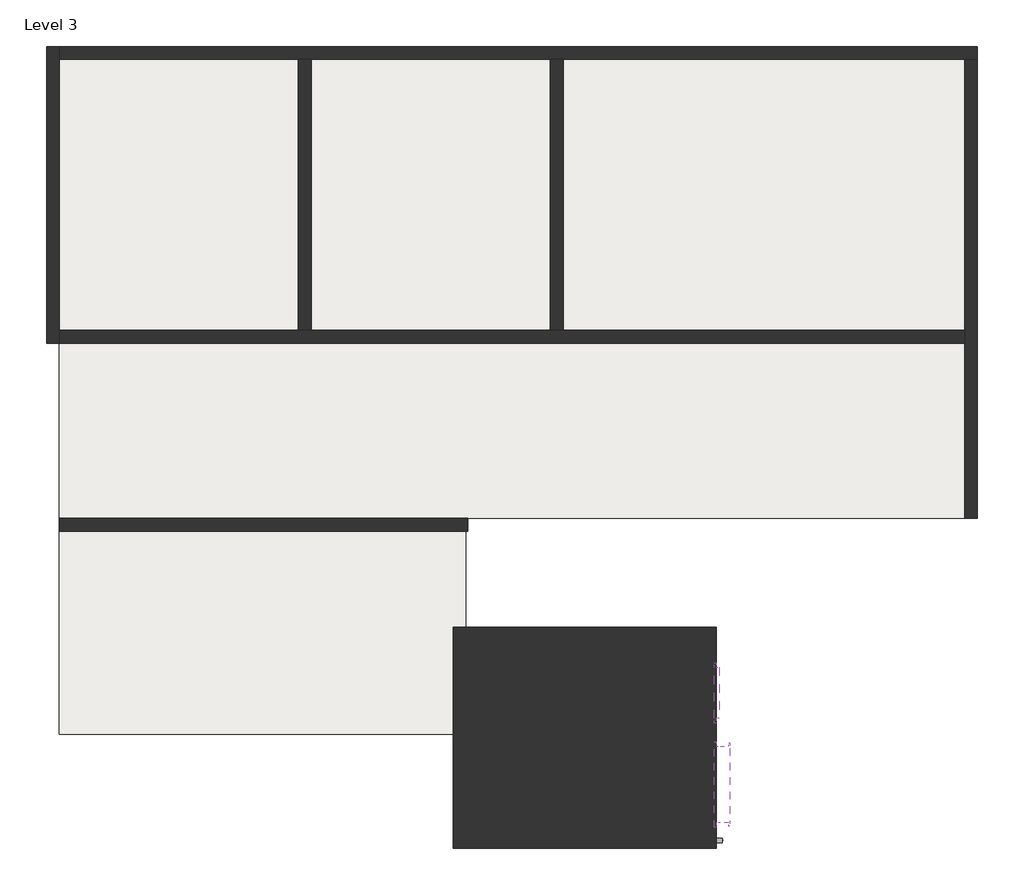
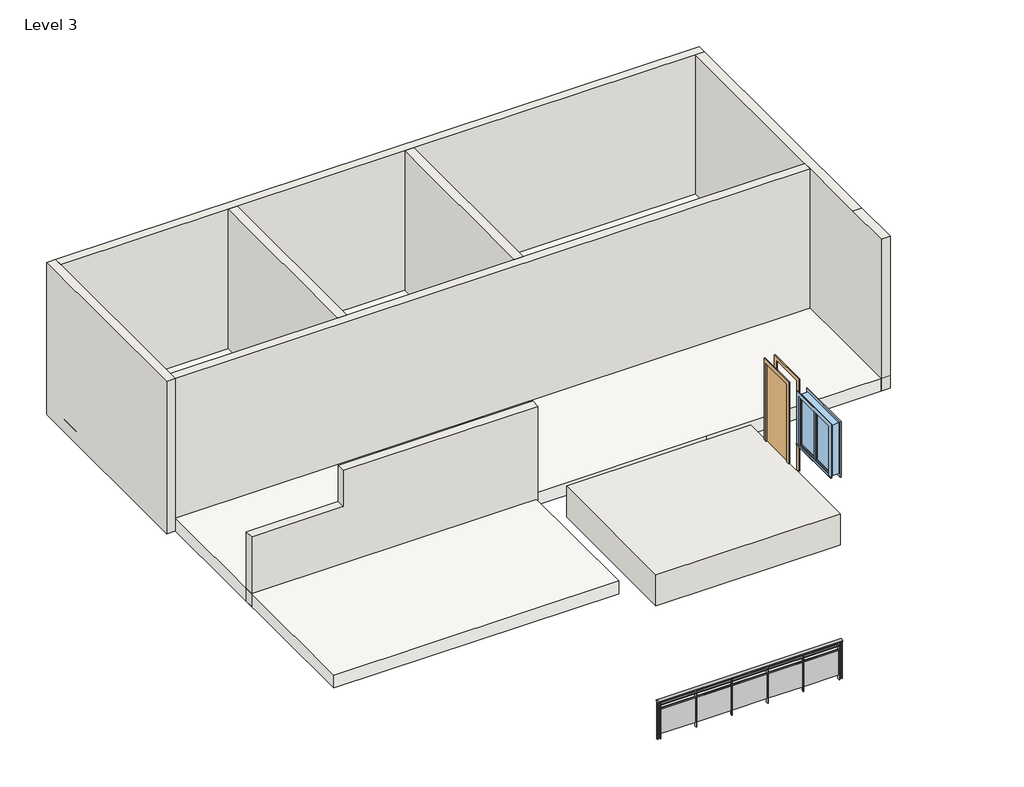
# One storey: 8 walls, 1 door, 1 railing, 1 roof, 1 window.
"""IFC4 building model written with IfcOpenShell, lengths in millimetres."""

from ifc_helpers import new_model, si_unit, point, frame, origin, place, context, project, spatial, polyline, ellipse_curve, trimmed, outline, extrude, faceted_brep, transform, mapped, element, save
from ifc_brep_helpers import plane_surface, extruded_surface, advanced_brep
from components import door_64d5ae29, walls_1_walls_1_cd3f7b89, window_0862ab64

model = new_model("IFC4")

# Units and contexts
model_context = context("Model", 3, world=origin())
ifc_project = project(units=[si_unit("LENGTHUNIT", "METRE", prefix="MILLI")], contexts=[model_context])

# Site, building, storey
site = spatial("IfcSite", under=ifc_project)
building = spatial("IfcBuilding", under=site)
storey = spatial("IfcBuildingStorey", under=building, Name="Level 3", Elevation=7315.2)

# Door
placement = place(None, origin())
door_shape = door_64d5ae29(model_context)
element("IfcDoor", 1, ObjectType="Single-Flush : 32\" x 84\"", at=placement, inside=storey, context=model_context, shape_type="MappedRepresentation", body=[
    mapped(door_shape, transform((-439.0620963, -2535.7885822, 8686.8), x_axis=(0.0, 1.0, 0.0), y_axis=(-1.0, 0.0, 0.0), z_axis=(0.0, 0.0, 1.0))),
])

# Railing
element("IfcRailing", 2, ObjectType="Glass Panel - Bottom Fill", at=placement, inside=storey, context=model_context, shape_type="SolidModel", body=[
    advanced_brep(
    [(-4630.0620963, -4847.1885822, 5791.2), (-4630.0620963, -4923.3885822, 5791.2), (-439.0620963, -4847.1885822, 5791.2), (-439.0620963, -4923.3885822, 5791.2)],
    [
        (0, 1, ellipse_curve(frame((-4630.0620963, -4885.2885822, 5791.2), z_axis=(-1.0, 0.0, 0.0), x_axis=(0.0, -1.0, 0.0)), 38.1, 28.575)),
        (1, 0, ellipse_curve(frame((-4630.0620963, -4885.2885822, 5791.2), z_axis=(-1.0, 0.0, 0.0), x_axis=(0.0, -1.0, 0.0)), 38.1, 28.575)),
        (2, 3, ellipse_curve(frame((-439.0620963, -4885.2885822, 5791.2), z_axis=(1.0, 0.0, 0.0), x_axis=(0.0, -1.0, 0.0)), 38.1, 28.575)),
        (3, 2, ellipse_curve(frame((-439.0620963, -4885.2885822, 5791.2), z_axis=(1.0, 0.0, 0.0), x_axis=(0.0, -1.0, 0.0)), 38.1, 28.575)),
        (0, 2),
        (3, 1),
    ],
    [
        plane_surface(frame((-4630.0620963, -4885.2885822, 5791.2), z_axis=(-1.0, 0.0, 0.0), x_axis=(0.0, 1.0, 0.0))),
        plane_surface(frame((-439.0620963, -4885.2885822, 5791.2), z_axis=(1.0, 0.0, 0.0), x_axis=(0.0, 1.0, 0.0))),
        extruded_surface(trimmed(ellipse_curve(frame((-439.0620963, -4885.2885822, 5791.2), z_axis=(-1.0, 0.0, 0.0), x_axis=(0.0, -1.0, 0.0)), 38.1, 28.575), [point((-439.0620963, -4847.1885822, 5791.2))], [point((-439.0620963, -4923.3885822, 5791.2))], True, "CARTESIAN"), (-4191.0, 0.0, 0.0), 4191.0),
        extruded_surface(trimmed(ellipse_curve(frame((-439.0620963, -4885.2885822, 5791.2), z_axis=(-1.0, 0.0, 0.0), x_axis=(0.0, -1.0, 0.0)), 38.1, 28.575), [point((-439.0620963, -4923.3885822, 5791.2))], [point((-439.0620963, -4847.1885822, 5791.2))], True, "CARTESIAN"), (-4191.0, 0.0, 0.0), 4191.0),
    ],
    [
        (0, [[1, 2]]),
        (1, [[3, 4]]),
        (2, [[-1, 5, -4, 6]]),
        (3, [[-2, -6, -3, -5]]),
    ],
),
    extrude(outline(polyline([(-4630.0620963, -4897.9885822), (-4630.0620963, -4872.5885822), (-439.0620963, -4872.5885822), (-439.0620963, -4897.9885822), (-4630.0620963, -4897.9885822)])), frame((0.0, 0.0, 5676.9), z_axis=(0.0, 0.0, 1.0), x_axis=(1.0, 0.0, 0.0)), (0.0, 0.0, 1.0), 25.4),
    extrude(outline(polyline([(-4630.0620963, -4897.9885822), (-4630.0620963, -4872.5885822), (-439.0620963, -4872.5885822), (-439.0620963, -4897.9885822), (-4630.0620963, -4897.9885822)])), frame((0.0, 0.0, 5575.3), z_axis=(0.0, 0.0, 1.0), x_axis=(1.0, 0.0, 0.0)), (0.0, 0.0, 1.0), 25.4),
    extrude(outline(polyline([(-508.9120963, -4910.6885822), (-508.9120963, -4859.8885822), (-496.2120963, -4859.8885822), (-496.2120963, -4910.6885822), (-508.9120963, -4910.6885822)])), frame((0.0, 0.0, 4876.8), z_axis=(0.0, 0.0, 1.0), x_axis=(1.0, 0.0, 0.0)), (0.0, 0.0, 1.0), 885.6788223),
    extrude(outline(polyline([(-1315.3620963, -4878.7534252), (-502.5620963, -4878.7534252), (-502.5620963, -4885.1034252), (-1315.3620963, -4885.1034252), (-1315.3620963, -4878.7534252)])), frame((0.0, 0.0, 4978.4), z_axis=(0.0, 0.0, 1.0), x_axis=(1.0, 0.0, 0.0)), (0.0, 0.0, 1.0), 596.9),
    extrude(outline(polyline([(-1321.7120963, -4910.6885822), (-1321.7120963, -4859.8885822), (-1309.0120963, -4859.8885822), (-1309.0120963, -4910.6885822), (-1321.7120963, -4910.6885822)])), frame((0.0, 0.0, 4876.8), z_axis=(0.0, 0.0, 1.0), x_axis=(1.0, 0.0, 0.0)), (0.0, 0.0, 1.0), 885.6788223),
    extrude(outline(polyline([(-2128.1620963, -4878.7534252), (-1315.3620963, -4878.7534252), (-1315.3620963, -4885.1034252), (-2128.1620963, -4885.1034252), (-2128.1620963, -4878.7534252)])), frame((0.0, 0.0, 4978.4), z_axis=(0.0, 0.0, 1.0), x_axis=(1.0, 0.0, 0.0)), (0.0, 0.0, 1.0), 596.9),
    extrude(outline(polyline([(-2134.5120963, -4910.6885822), (-2134.5120963, -4859.8885822), (-2121.8120963, -4859.8885822), (-2121.8120963, -4910.6885822), (-2134.5120963, -4910.6885822)])), frame((0.0, 0.0, 4876.8), z_axis=(0.0, 0.0, 1.0), x_axis=(1.0, 0.0, 0.0)), (0.0, 0.0, 1.0), 885.6788223),
    extrude(outline(polyline([(-2940.9620963, -4878.7534252), (-2128.1620963, -4878.7534252), (-2128.1620963, -4885.1034252), (-2940.9620963, -4885.1034252), (-2940.9620963, -4878.7534252)])), frame((0.0, 0.0, 4978.4), z_axis=(0.0, 0.0, 1.0), x_axis=(1.0, 0.0, 0.0)), (0.0, 0.0, 1.0), 596.9),
    extrude(outline(polyline([(-2947.3120963, -4910.6885822), (-2947.3120963, -4859.8885822), (-2934.6120963, -4859.8885822), (-2934.6120963, -4910.6885822), (-2947.3120963, -4910.6885822)])), frame((0.0, 0.0, 4876.8), z_axis=(0.0, 0.0, 1.0), x_axis=(1.0, 0.0, 0.0)), (0.0, 0.0, 1.0), 885.6788223),
    extrude(outline(polyline([(-3753.7620963, -4878.7534252), (-2940.9620963, -4878.7534252), (-2940.9620963, -4885.1034252), (-3753.7620963, -4885.1034252), (-3753.7620963, -4878.7534252)])), frame((0.0, 0.0, 4978.4), z_axis=(0.0, 0.0, 1.0), x_axis=(1.0, 0.0, 0.0)), (0.0, 0.0, 1.0), 596.9),
    extrude(outline(polyline([(-3760.1120963, -4910.6885822), (-3760.1120963, -4859.8885822), (-3747.4120963, -4859.8885822), (-3747.4120963, -4910.6885822), (-3760.1120963, -4910.6885822)])), frame((0.0, 0.0, 4876.8), z_axis=(0.0, 0.0, 1.0), x_axis=(1.0, 0.0, 0.0)), (0.0, 0.0, 1.0), 885.6788223),
    extrude(outline(polyline([(-4566.5620963, -4878.7534252), (-3753.7620963, -4878.7534252), (-3753.7620963, -4885.1034252), (-4566.5620963, -4885.1034252), (-4566.5620963, -4878.7534252)])), frame((0.0, 0.0, 4978.4), z_axis=(0.0, 0.0, 1.0), x_axis=(1.0, 0.0, 0.0)), (0.0, 0.0, 1.0), 596.9),
    extrude(outline(polyline([(-4572.9120963, -4910.6885822), (-4572.9120963, -4859.8885822), (-4560.2120963, -4859.8885822), (-4560.2120963, -4910.6885822), (-4572.9120963, -4910.6885822)])), frame((0.0, 0.0, 4876.8), z_axis=(0.0, 0.0, 1.0), x_axis=(1.0, 0.0, 0.0)), (0.0, 0.0, 1.0), 885.6788223),
    extrude(outline(polyline([(-451.7620963, -4894.8135822), (-451.7620963, -4875.7635822), (-432.7120963, -4875.7635822), (-432.7120963, -4894.8135822), (-451.7620963, -4894.8135822)])), frame((0.0, 0.0, 4876.8), z_axis=(0.0, 0.0, 1.0), x_axis=(1.0, 0.0, 0.0)), (0.0, 0.0, 1.0), 885.6788223),
    extrude(outline(polyline([(-4636.4120963, -4894.8135822), (-4636.4120963, -4875.7635822), (-4617.3620963, -4875.7635822), (-4617.3620963, -4894.8135822), (-4636.4120963, -4894.8135822)])), frame((0.0, 0.0, 4876.8), z_axis=(0.0, 0.0, 1.0), x_axis=(1.0, 0.0, 0.0)), (0.0, 0.0, 1.0), 885.6788223),
])

# Roof
element("IfcRoof", 3, ObjectType="Generic - 12\"", at=placement, inside=storey, context=model_context, shape_type="SweptSolid", body=[
    extrude(outline(polyline([(-11208.6620963, 7763.9114178), (3624.9379037, 7763.9114178), (3624.9379037, 245.5114178), (-540.6620963, 245.5114178), (-4528.4620963, 245.5114178), (-4528.4620963, -3196.1885822), (-11005.4620963, -3196.1885822), (-11005.4620963, 3039.5114178), (-11208.6620963, 3039.5114178), (-11208.6620963, 7763.9114178)])), frame((0.0, 0.0, 7315.2), z_axis=(0.0, 0.0, 1.0), x_axis=(1.0, 0.0, 0.0)), (0.0, 0.0, 1.0), 304.8),
])

# Walls
element("IfcWall", 4, ObjectType="Generic - 8\"", at=placement, inside=storey, context=model_context, shape_type="Brep", body=[
    faceted_brep([(-11208.6620963, 7763.9114178, 7315.2), (-11208.6620963, 3039.5114178, 7315.2), (-11208.6620963, 3039.5114178, 10972.8), (-11208.6620963, 7763.9114178, 10972.8), (-11005.4620963, 7763.9114178, 7315.2), (-11005.4620963, 7763.9114178, 10972.8), (-11005.4620963, 7560.7114178, 10972.8), (-11005.4620963, 3242.7114178, 10972.8), (-11005.4620963, 3039.5114178, 10972.8), (-11005.4620963, 3039.5114178, 7315.2), (-11005.4620963, 3242.7114178, 7315.2), (-11005.4620963, 7560.7114178, 7315.2)], [[[0, 1, 2, 3]], [[4, 5, 6, 7, 8, 9, 10, 11]], [[1, 0, 4, 11, 10, 9]], [[0, 3, 5, 4]], [[2, 1, 9, 8]], [[3, 2, 8, 7, 6, 5]]]),
])
element("IfcWall", 5, ObjectType="Generic - 8\"", at=placement, inside=storey, context=model_context, shape_type="Brep", body=[
    faceted_brep([(-11005.4620963, 7560.7114178, 7315.2), (-7195.4620963, 7560.7114178, 7315.2), (-6992.2620963, 7560.7114178, 7315.2), (-3182.2620963, 7560.7114178, 7315.2), (-2979.0620963, 7560.7114178, 7315.2), (3421.7379037, 7560.7114178, 7315.2), (3624.9379037, 7560.7114178, 7315.2), (3624.9379037, 7560.7114178, 10972.8), (3421.7379037, 7560.7114178, 10972.8), (-2979.0620963, 7560.7114178, 10972.8), (-3182.2620963, 7560.7114178, 10972.8), (-6992.2620963, 7560.7114178, 10972.8), (-7195.4620963, 7560.7114178, 10972.8), (-11005.4620963, 7560.7114178, 10972.8), (-11005.4620963, 7763.9114178, 7315.2), (-11005.4620963, 7763.9114178, 10972.8), (3624.9379037, 7763.9114178, 10972.8), (3624.9379037, 7763.9114178, 7315.2)], [[[0, 1, 2, 3, 4, 5, 6, 7, 8, 9, 10, 11, 12, 13]], [[14, 15, 16, 17]], [[6, 5, 4, 3, 2, 1, 0, 14, 17]], [[0, 13, 15, 14]], [[7, 6, 17, 16]], [[13, 12, 11, 10, 9, 8, 7, 16, 15]]]),
])
element("IfcWall", 6, ObjectType="Generic - 8\"", at=placement, inside=storey, context=model_context, shape_type="Brep", body=[
    faceted_brep([(3421.7379037, 7560.7114178, 7315.2), (3421.7379037, 3242.7114178, 7315.2), (3421.7379037, 3039.5114178, 7315.2), (3421.7379037, 245.5114178, 7315.2), (3421.7379037, 245.5114178, 10972.8), (3421.7379037, 1363.1114178, 10972.8), (3421.7379037, 3039.5114178, 10972.8), (3421.7379037, 3242.7114178, 10972.8), (3421.7379037, 7560.7114178, 10972.8), (3624.9379037, 7560.7114178, 7315.2), (3624.9379037, 7560.7114178, 10972.8), (3624.9379037, 1363.1114178, 10972.8), (3624.9379037, 245.5114178, 10972.8), (3624.9379037, 245.5114178, 7315.2)], [[[0, 1, 2, 3, 4, 5, 6, 7, 8]], [[9, 10, 11, 12, 13]], [[3, 2, 1, 0, 9, 13]], [[4, 3, 13, 12]], [[0, 8, 10, 9]], [[5, 4, 12, 11]], [[8, 7, 6, 5, 11, 10]]]),
])
element("IfcWall", 7, ObjectType="Generic - 8\"", at=placement, inside=storey, context=model_context, shape_type="Brep", body=[
    faceted_brep([(-11005.4620963, 3039.5114178, 7315.2), (3421.7379037, 3039.5114178, 7315.2), (3421.7379037, 3039.5114178, 10972.8), (-11005.4620963, 3039.5114178, 10972.8), (-11005.4620963, 3242.7114178, 7315.2), (-11005.4620963, 3242.7114178, 10972.8), (-7195.4620963, 3242.7114178, 10972.8), (-6992.2620963, 3242.7114178, 10972.8), (-3182.2620963, 3242.7114178, 10972.8), (-2979.0620963, 3242.7114178, 10972.8), (3421.7379037, 3242.7114178, 10972.8), (3421.7379037, 3242.7114178, 7315.2), (-2979.0620963, 3242.7114178, 7315.2), (-3182.2620963, 3242.7114178, 7315.2), (-6992.2620963, 3242.7114178, 7315.2), (-7195.4620963, 3242.7114178, 7315.2)], [[[0, 1, 2, 3]], [[4, 5, 6, 7, 8, 9, 10, 11, 12, 13, 14, 15]], [[1, 0, 4, 15, 14, 13, 12, 11]], [[0, 3, 5, 4]], [[2, 1, 11, 10]], [[3, 2, 10, 9, 8, 7, 6, 5]]]),
])
element("IfcWall", 8, ObjectType="Generic - 8\"", at=placement, inside=storey, context=model_context, shape_type="SweptSolid", body=[
    extrude(outline(polyline([(-6992.2620963, 7560.7114178), (-6992.2620963, 3242.7114178), (-7195.4620963, 3242.7114178), (-7195.4620963, 7560.7114178), (-6992.2620963, 7560.7114178)])), frame((0.0, 0.0, 7315.2), z_axis=(0.0, 0.0, 1.0), x_axis=(1.0, 0.0, 0.0)), (0.0, 0.0, 1.0), 3657.6),
])
element("IfcWall", 9, ObjectType="Generic - 8\"", at=placement, inside=storey, context=model_context, shape_type="SweptSolid", body=[
    extrude(outline(polyline([(-2979.0620963, 7560.7114178), (-2979.0620963, 3242.7114178), (-3182.2620963, 3242.7114178), (-3182.2620963, 7560.7114178), (-2979.0620963, 7560.7114178)])), frame((0.0, 0.0, 7315.2), z_axis=(0.0, 0.0, 1.0), x_axis=(1.0, 0.0, 0.0)), (0.0, 0.0, 1.0), 3657.6),
])
element("IfcWall", 10, ObjectType="Generic - 8\"", at=placement, inside=storey, context=model_context, shape_type="Brep", body=[
    faceted_brep([(-11005.4620963, 42.3114178, 7315.2), (-4496.7120963, 42.3114178, 7315.2), (-4496.7120963, 42.3114178, 9847.8766226), (-8922.6620963, 42.3114178, 9847.8766226), (-8922.6620963, 42.3114178, 8984.2766226), (-11005.4620963, 42.3114178, 8984.2766226), (-11005.4620963, 245.5114178, 7315.2), (-11005.4620963, 245.5114178, 8977.6089989), (-11005.4620963, 245.5114178, 8984.2766226), (-8922.6620963, 245.5114178, 8984.2766226), (-8922.6620963, 245.5114178, 9847.8766226), (-4496.7120963, 245.5114178, 9847.8766226), (-4496.7120963, 245.5114178, 7315.2)], [[[0, 1, 2, 3, 4, 5]], [[6, 7, 8, 9, 10, 11, 12]], [[0, 5, 8, 7, 6]], [[1, 0, 6, 12]], [[2, 1, 12, 11]], [[3, 2, 11, 10]], [[4, 3, 10, 9]], [[5, 4, 9, 8]]]),
])
walls_1_walls_1_shape = walls_1_walls_1_cd3f7b89(model_context)
element("IfcWall", 11, ObjectType="Walls 1 : Walls 1", at=placement, inside=storey, context=model_context, shape_type="MappedRepresentation", body=[
    mapped(walls_1_walls_1_shape, transform((0.0, 0.0, 0.0), x_axis=(1.0, 0.0, 0.0), y_axis=(0.0, 1.0, 0.0), z_axis=(0.0, 0.0, 1.0))),
])

# Window
window_shape = window_0862ab64(model_context)
element("IfcWindow", 12, ObjectType="Casement Dbl with Trim.0001 : 48\" x 48\"", at=placement, inside=storey, context=model_context, shape_type="MappedRepresentation", body=[
    mapped(window_shape, transform((-420.0120963, -3996.2885822, 8680.5318944), x_axis=(0.0, 1.0, 0.0), y_axis=(-1.0, 0.0, 0.0), z_axis=(0.0, 0.0, 1.0))),
])

save(model, "model.ifc")

# Revit data of these elements
# Type "Single-Flush : 32\" x 84\""
#   Type Mark = "3"
#   Construction Type Id = "MDOOR"
#   Assembly Code = "C1020"
#   Analytic Construction = "Metal"
#   Thickness = 0' - 2"
#   Heat Transfer Coefficient (U) = 0.651978 BTU/(h·ft²·°F)
#   Height = 7' - 0"
#   Trim Projection Ext = 0' - 1"
#   Trim Projection Int = 0' - 1"
#   Trim Width = 0' - 3"
#   Width = 2' - 8"
#   Define Thermal Properties by = 1
#   Door Material = Door - Panel
#   Frame Material = Door - Frame
#   Visual Light Transmittance = 0
#   Solar Heat Gain Coefficient = 0
#   Function = (empty or 0)
#   Wall Closure = (empty or 0)
# Type "Glass Panel - Bottom Fill"
#   Assembly Code = "C2010400"
#   built-in parameter 1008612 = 0.0416667 (stored number, unit not read)
#   built-in parameter 1008611 = 0.0416667 (stored number, unit not read)
#   built-in parameter 1008609 = 0.333333 (stored number, unit not read)
#   built-in parameter 1008604 = 0.166667 (stored number, unit not read)
#   built-in parameter 1008603 = 0.166667 (stored number, unit not read)
#   Railing Height = 3' - 0"
#   built-in parameter 1008630 = 2
#   built-in parameter 1008610 = 2
#   built-in parameter 1008618 = Baluster - Square : 3/4"
# Type "Generic - 12\""
#   Assembly Code = "B1020"
#   Layers, outside or top first: 1' - 0" no material (function 1)
# Type "Generic - 8\""
#   Assembly Code = "B2010"
#   Layers, outside or top first: 0' - 8" no material (function 1)
# Type "Casement Dbl with Trim.0001 : 48\" x 48\""
#   Type Mark = "10"
#   Construction Type Id = "GSP4R"
#   Assembly Code = "B2020100"
#   Analytic Construction = "1/8 in Pilkington single glazing"
#   Visual Light Transmittance = 0.9
#   Solar Heat Gain Coefficient = 0.78
#   Heat Transfer Coefficient (U) = 0.6496 BTU/(h·ft²·°F)
#   Height = 4' - 0"
#   Default Sill Height = 3' - 0"
#   Trim Projection - Ext. = 0' - 0 1/2"
#   Trim Projection - Int. = 0' - 0 3/4"
#   Trim Width - Exterior = 0' - 3 1/2"
#   Trim Width - Interior = 0' - 3 1/2"
#   Width = 4' - 0"
#   Window Inset = 0' - 0 3/4"
#   Define Thermal Properties by = 1
#   Glass Pane Material = Glass
#   Sash Material = Sash
#   Trim Exterior Material = Trim
#   Trim Interior Material = Trim
#   Wall Closure = (empty or 0)
# Element 1 (IfcDoor, "Single-Flush : 32\" x 84\"")
#   Phase Created = New Construction
#   Materials on its faces: "Door - Frame", "Door - Panel"
# Element 2 (IfcRailing, "Glass Panel - Bottom Fill")
#   built-in parameter 1008621 = -8 (stored number, unit not read)
#   Phase Created = New Construction
#   Materials on its faces: "Glass"
# Element 3 (IfcRoof, "Generic - 12\"")
#   built-in parameter 1001705 = 25 (stored number, unit not read)
#   built-in parameter 1001710 = 33615
#   Phase Created = New Construction
#   Materials on its faces: "Default Roof"
# Elements 4, 5, 6, 7, 8, 9 (IfcWall, "Generic - 8\"")
#   Top Offset = 0' - 0"
#   Base Offset = 0' - 0"
#   Unconnected Height = 12' - 0"
#   wall height = 12' - 0"
#   Phase Created = New Construction
#   Base Constraint = Level 3
#   Materials on its faces: "Default Wall"
# Element 10 (IfcWall, "Generic - 8\"")
#   Top Offset = 0' - 0"
#   Base Offset = 0' - 0"
#   Unconnected Height = 8' - 3.71168"
#   wall height = 8' - 3.71168"
#   Phase Created = New Construction
#   Base Constraint = Level 3
#   Materials on its faces: "Default Wall"
# Element 11 (IfcWall, "Walls 1 : Walls 1")
#   Phase Created = New Construction
#   Materials on its faces: "Default Wall"
# Element 12 (IfcWindow, "Casement Dbl with Trim.0001 : 48\" x 48\"")
#   Mark = "4"
#   Phase Created = New Construction
#   Materials on its faces: "Sash", "Trim", "Glass"
# Materials
#   "Door - Panel": class "Wood", colour RGB 210 159 95, transparency 0
#   "Door - Frame": colour RGB 118 70 51, transparency 0
#   "Glass": class "Glass", colour RGB 0 128 192, transparency 0.75, Description = "Soda Lime Glass", Cost = 0
#   "Sash": class "Wood", colour RGB 224 178 126, transparency 0
#   "Trim": class "Wood", colour RGB 224 178 126, transparency 0
#   "Default Roof": colour RGB 88 101 114, transparency 0
#   "Default Wall": colour RGB 128 128 128, transparency 0
